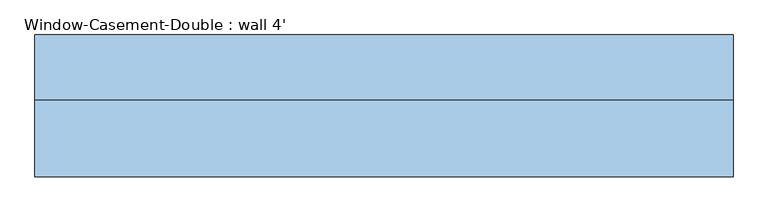
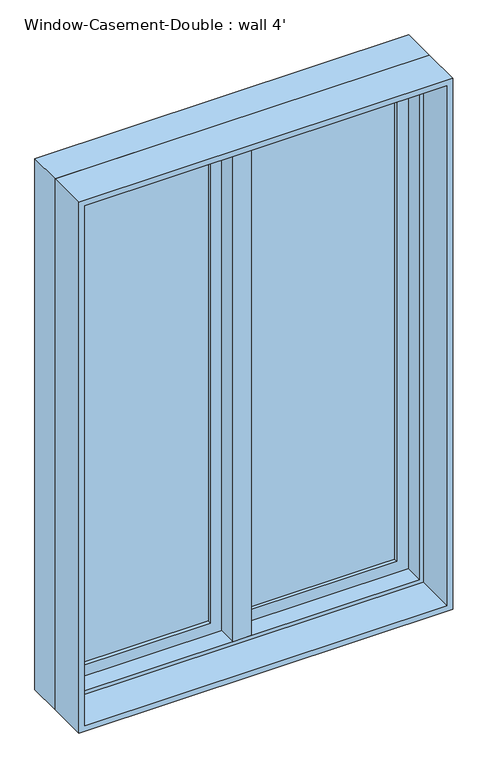
"""IFC4 building model written with IfcOpenShell, lengths in millimetres: window geometry, Window-Casement-Double : wall 4'."""

from ifc_helpers import new_model, si_unit, frame, origin, place, context, project, spatial, polyline, outline, extrude, faceted_brep, source, transform, mapped, element, save


def window_casement_double_wall_4_6ca1769e(model_context):
    return source(origin(), model_context, "Body", "SolidModel", [
        faceted_brep([(9.525, 133.35, 2730.5), (-9.525, 133.35, 2730.5), (-9.525, 82.55, 2730.5), (9.525, 82.55, 2730.5), (9.525, 133.35, 927.1), (9.525, 82.55, 927.1), (-9.525, 82.55, 927.1), (-9.525, 133.35, 927.1), (-9.525, 82.55, 946.15), (-9.525, 82.55, 2711.45), (-30.1625, 82.55, 946.15), (-30.1625, 82.55, 2711.45), (-30.1625, 19.05, 946.15), (-30.1625, 19.05, 2711.45), (30.1625, 19.05, 946.15), (30.1625, 19.05, 2711.45), (30.1625, 82.55, 946.15), (30.1625, 82.55, 2711.45), (9.525, 82.55, 946.15), (9.525, 82.55, 2711.45)], [[[0, 1, 2, 3]], [[4, 5, 6, 7]], [[1, 0, 4, 7]], [[2, 1, 7, 6, 8, 9]], [[9, 8, 10, 11]], [[11, 10, 12, 13]], [[13, 12, 14, 15]], [[15, 14, 16, 17]], [[17, 16, 18, 19]], [[0, 3, 19, 18, 5, 4]], [[18, 8, 6, 5]], [[9, 19, 3, 2]], [[8, 18, 16, 14, 12, 10]], [[19, 9, 11, 13, 15, 17]]]),
        extrude(outline(polyline([(-66.675, 114.3), (-66.675, 107.95), (-539.75, 107.95), (-539.75, 114.3), (-66.675, 114.3)])), frame((0.0, 0.0, 984.25), z_axis=(0.0, 0.0, 1.0), x_axis=(1.0, 0.0, 0.0)), (0.0, 0.0, 1.0), 1689.1),
        extrude(outline(polyline([(-539.75, 95.25), (-539.75, 101.6), (-66.675, 101.6), (-66.675, 95.25), (-539.75, 95.25)])), frame((0.0, 0.0, 984.25), z_axis=(0.0, 0.0, 1.0), x_axis=(1.0, 0.0, 0.0)), (0.0, 0.0, 1.0), 1689.1),
        extrude(outline(polyline([(539.75, 114.3), (539.75, 107.95), (66.675, 107.95), (66.675, 114.3), (539.75, 114.3)])), frame((0.0, 0.0, 984.25), z_axis=(0.0, 0.0, 1.0), x_axis=(1.0, 0.0, 0.0)), (0.0, 0.0, 1.0), 1689.1),
        extrude(outline(polyline([(66.675, 95.25), (66.675, 101.6), (539.75, 101.6), (539.75, 95.25), (66.675, 95.25)])), frame((0.0, 0.0, 984.25), z_axis=(0.0, 0.0, 1.0), x_axis=(1.0, 0.0, 0.0)), (0.0, 0.0, 1.0), 1689.1),
        extrude(outline(polyline([(2730.5, -596.9), (927.1, -596.9), (927.1, -9.525), (2730.5, -9.525), (2730.5, -596.9)]), holes=[polyline([(2673.35, -66.675), (984.25, -66.675), (984.25, -539.75), (2673.35, -539.75), (2673.35, -66.675)])]), frame((0.0, 82.55, 0.0), z_axis=(0.0, 1.0, 0.0), x_axis=(0.0, 0.0, 1.0)), (0.0, 0.0, 1.0), 44.45),
        extrude(outline(polyline([(927.1, 596.9), (2730.5, 596.9), (2730.5, 9.525), (927.1, 9.525), (927.1, 596.9)]), holes=[polyline([(984.25, 66.675), (2673.35, 66.675), (2673.35, 539.75), (984.25, 539.75), (984.25, 66.675)])]), frame((0.0, 82.55, 0.0), z_axis=(0.0, 1.0, 0.0), x_axis=(0.0, 0.0, 1.0)), (0.0, 0.0, 1.0), 44.45),
        extrude(outline(polyline([(2743.2, -609.6), (914.4, -609.6), (914.4, 609.6), (2743.2, 609.6), (2743.2, -609.6)]), holes=[polyline([(2724.15, 590.55), (933.45, 590.55), (933.45, -590.55), (2724.15, -590.55), (2724.15, 590.55)])]), frame((0.0, -114.3, 0.0), z_axis=(0.0, 1.0, 0.0), x_axis=(0.0, 0.0, 1.0)), (0.0, 0.0, 1.0), 133.35),
        faceted_brep([(577.85, 82.55, 2711.45), (577.85, 19.05, 2711.45), (-577.85, 19.05, 2711.45), (-577.85, 82.55, 2711.45), (596.9, 133.35, 2730.5), (596.9, 82.55, 2730.5), (-596.9, 82.55, 2730.5), (-596.9, 133.35, 2730.5), (609.6, 19.05, 2743.2), (609.6, 133.35, 2743.2), (-609.6, 133.35, 2743.2), (-609.6, 19.05, 2743.2), (-577.85, 19.05, 946.15), (-577.85, 82.55, 946.15), (-596.9, 82.55, 927.1), (-596.9, 133.35, 927.1), (-609.6, 133.35, 914.4), (-609.6, 19.05, 914.4), (577.85, 19.05, 946.15), (577.85, 82.55, 946.15), (596.9, 82.55, 927.1), (596.9, 133.35, 927.1), (609.6, 133.35, 914.4), (609.6, 19.05, 914.4)], [[[0, 1, 2, 3]], [[4, 5, 6, 7]], [[8, 9, 10, 11]], [[3, 2, 12, 13]], [[7, 6, 14, 15]], [[11, 10, 16, 17]], [[13, 12, 18, 19]], [[15, 14, 20, 21]], [[17, 16, 22, 23]], [[11, 17, 23, 8], [1, 18, 12, 2]], [[19, 18, 1, 0]], [[5, 20, 14, 6], [3, 13, 19, 0]], [[21, 20, 5, 4]], [[23, 22, 9, 8]], [[9, 22, 16, 10], [7, 15, 21, 4]]]),
    ])


if __name__ == "__main__":
    model = new_model("IFC4")
    model_context = context("Model", 3, world=origin())
    ifc_project = project(units=[si_unit("LENGTHUNIT", "METRE", prefix="MILLI")], contexts=[model_context])
    site = spatial("IfcSite", under=ifc_project)
    building = spatial("IfcBuilding", under=site)
    placement = place(None, origin())
    window_casement_double_wall_4_shape = window_casement_double_wall_4_6ca1769e(model_context)
    element("IfcWindow", 1, ObjectType="Window-Casement-Double : wall 4'", at=placement, inside=building, context=model_context, shape_type="MappedRepresentation", body=[
        mapped(window_casement_double_wall_4_shape, transform((0.0, 0.0, 0.0), x_axis=(1.0, 0.0, 0.0), y_axis=(0.0, 1.0, 0.0), z_axis=(0.0, 0.0, 1.0))),
    ])
    save(model, "model.ifc")

# Revit data of these elements
# Type "Window-Casement-Double : wall 4'"
#   Type Mark = "19"
#   Fire Rating = "0.5h"
#   Assembly Code = "B2020100"
#   Analytic Construction = "Double glazing - domestic"
#   Frame Extension [instance default] = 0' - 0 1/4"
#   Window Inset [instance default] = 0' - 0"
#   Wall Thickness [instance default] = 0' - 6"
#   Interior Wall Closure [instance default] = 0' - 2 1/4"
#   Half Width = 2' - 0"
#   Visual Light Transmittance = 0.81
#   Thermal Resistance (R) = 1.8146 (h·ft²·°F)/BTU
#   Solar Heat Gain Coefficient = 0.76
#   Rough Width = 4' - 0 1/2"
#   Rough Height = 6' - 0 1/2"
#   Height = 6' - 0"
#   Heat Transfer Coefficient (U) = 0.5511 BTU/(h·ft²·°F)
#   Exterior Wall Closure [instance default] = 0' - 1 1/4"
#   Extension Jamb [instance default] = 0' - 2 1/4"
#   Default Sill Height = 3' - 0"
#   Width = 4' - 0"
#   Muntin Visibility = yes
#   Interior Trim Visibility [instance default] = yes
#   Exterior Trim Visibility [instance default] = yes
#   Extension Jamb Visibility [instance default] = yes
#   Interior Trim Material = Wood - Stained
#   Muntin Pattern = Muntin Pattern_2x2 : Muntin Pattern_2x2
#   Interior Trim = Trim-Window-Interior-Flat : Picture Frame
#   Interior Frame Material = Wood - Stained
#   Glass Panel Material = Glass
#   Exterior Trim Material = Clad - White
#   Exterior Trim = Trim-Window-Exterior-Flat : with Sill
#   Exterior Frame Material = Clad - White
#   Wall Closure = (empty or 0)
# Element 1 (IfcWindow, "Window-Casement-Double : wall 4'")
#   Wall Thickness = 0' - 9"
#   Extension Jamb = 0' - 5 1/4"
#   Materials on its faces: "Wood - Stained", "Glass", "Clad - White"
# Materials
#   "Wood - Stained": class "Wood", colour RGB 224 178 126, transparency 0, Cost = 0
#   "Glass": class "Glass", colour RGB 0 128 192, transparency 0.75, Description = "Soda Lime Glass", Cost = 0
#   "Clad - White": class "Wood", colour RGB 242 242 238, transparency 0, Cost = 0
